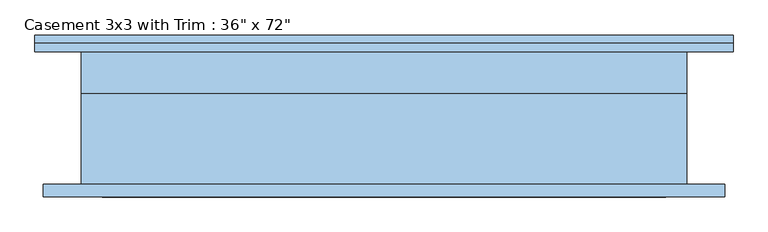
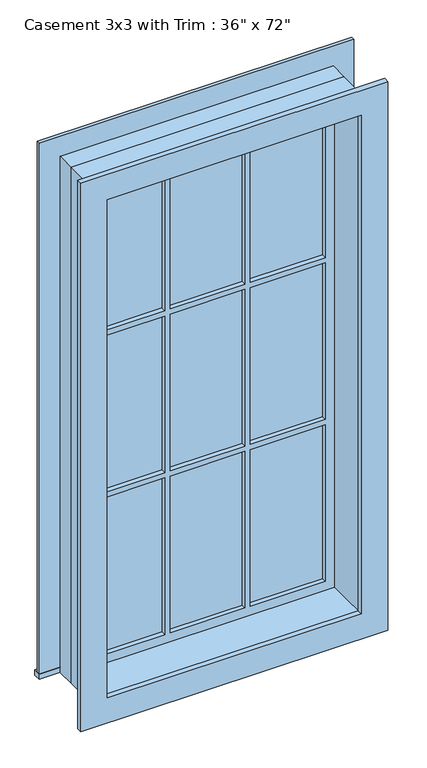
"""IFC4 building model written with IfcOpenShell, lengths in millimetres: window geometry."""

from ifc_helpers import new_model, si_unit, frame, origin, place, context, project, spatial, polyline, outline, extrude, source, transform, mapped, element, save


def window_0c844ac8(model_context):
    return source(origin(), model_context, "Body", "SweptSolid", [
        extrude(outline(polyline([(-527.05, 125.4), (527.05, 125.4), (527.05, 100.0), (-527.05, 100.0), (-527.05, 125.4)])), frame((0.0, 0.0, 304.8), z_axis=(0.0, 0.0, 1.0), x_axis=(1.0, 0.0, 0.0)), (0.0, 0.0, 1.0), 19.05),
        extrude(outline(polyline([(2114.55, -438.15), (2114.55, 438.15), (323.85, 438.15), (323.85, 527.05), (2203.45, 527.05), (2203.45, -527.05), (323.85, -527.05), (323.85, -438.15), (2114.55, -438.15)])), frame((0.0, 100.0, 0.0), z_axis=(0.0, 1.0, 0.0), x_axis=(0.0, 0.0, 1.0)), (0.0, 0.0, 1.0), 12.7),
        extrude(outline(polyline([(143.9333333, 65.075), (393.7, 65.075), (393.7, 52.375), (143.9333333, 52.375), (143.9333333, 65.075)])), frame((0.0, 0.0, 1515.5333333), z_axis=(0.0, 0.0, 1.0), x_axis=(1.0, 0.0, 0.0)), (0.0, 0.0, 1.0), 554.5666667),
        extrude(outline(polyline([(-124.8833333, 65.075), (124.8833333, 65.075), (124.8833333, 52.375), (-124.8833333, 52.375), (-124.8833333, 65.075)])), frame((0.0, 0.0, 1515.5333333), z_axis=(0.0, 0.0, 1.0), x_axis=(1.0, 0.0, 0.0)), (0.0, 0.0, 1.0), 554.5666667),
        extrude(outline(polyline([(-393.7, 65.075), (-143.9333333, 65.075), (-143.9333333, 52.375), (-393.7, 52.375), (-393.7, 65.075)])), frame((0.0, 0.0, 1515.5333333), z_axis=(0.0, 0.0, 1.0), x_axis=(1.0, 0.0, 0.0)), (0.0, 0.0, 1.0), 554.5666667),
        extrude(outline(polyline([(-393.7, 65.075), (-143.9333333, 65.075), (-143.9333333, 52.375), (-393.7, 52.375), (-393.7, 65.075)])), frame((0.0, 0.0, 941.9166667), z_axis=(0.0, 0.0, 1.0), x_axis=(1.0, 0.0, 0.0)), (0.0, 0.0, 1.0), 554.5666667),
        extrude(outline(polyline([(-124.8833333, 65.075), (124.8833333, 65.075), (124.8833333, 52.375), (-124.8833333, 52.375), (-124.8833333, 65.075)])), frame((0.0, 0.0, 941.9166667), z_axis=(0.0, 0.0, 1.0), x_axis=(1.0, 0.0, 0.0)), (0.0, 0.0, 1.0), 554.5666667),
        extrude(outline(polyline([(143.9333333, 65.075), (393.7, 65.075), (393.7, 52.375), (143.9333333, 52.375), (143.9333333, 65.075)])), frame((0.0, 0.0, 941.9166667), z_axis=(0.0, 0.0, 1.0), x_axis=(1.0, 0.0, 0.0)), (0.0, 0.0, 1.0), 554.5666667),
        extrude(outline(polyline([(143.9333333, 65.075), (393.7, 65.075), (393.7, 52.375), (143.9333333, 52.375), (143.9333333, 65.075)])), frame((0.0, 0.0, 368.3), z_axis=(0.0, 0.0, 1.0), x_axis=(1.0, 0.0, 0.0)), (0.0, 0.0, 1.0), 554.5666667),
        extrude(outline(polyline([(-124.8833333, 65.075), (124.8833333, 65.075), (124.8833333, 52.375), (-124.8833333, 52.375), (-124.8833333, 65.075)])), frame((0.0, 0.0, 368.3), z_axis=(0.0, 0.0, 1.0), x_axis=(1.0, 0.0, 0.0)), (0.0, 0.0, 1.0), 554.5666667),
        extrude(outline(polyline([(-393.7, 65.075), (-143.9333333, 65.075), (-143.9333333, 52.375), (-393.7, 52.375), (-393.7, 65.075)])), frame((0.0, 0.0, 368.3), z_axis=(0.0, 0.0, 1.0), x_axis=(1.0, 0.0, 0.0)), (0.0, 0.0, 1.0), 554.5666667),
        extrude(outline(polyline([(2190.75, 514.35), (2190.75, -514.35), (247.65, -514.35), (247.65, 514.35), (2190.75, 514.35)]), holes=[polyline([(2101.85, 425.45), (336.55, 425.45), (336.55, -425.45), (2101.85, -425.45), (2101.85, 425.45)])]), frame((0.0, -119.05, 0.0), z_axis=(0.0, 1.0, 0.0), x_axis=(0.0, 0.0, 1.0)), (0.0, 0.0, 1.0), 19.05),
        extrude(outline(polyline([(2114.55, -438.15), (323.85, -438.15), (323.85, 438.15), (2114.55, 438.15), (2114.55, -438.15)]), holes=[polyline([(2070.1, -143.9333333), (1515.5333333, -143.9333333), (1515.5333333, -393.7), (2070.1, -393.7), (2070.1, -143.9333333)]), polyline([(1496.4833333, -143.9333333), (941.9166667, -143.9333333), (941.9166667, -393.7), (1496.4833333, -393.7), (1496.4833333, -143.9333333)]), polyline([(922.8666667, -143.9333333), (368.3, -143.9333333), (368.3, -393.7), (922.8666667, -393.7), (922.8666667, -143.9333333)]), polyline([(2070.1, 124.8833333), (1515.5333333, 124.8833333), (1515.5333333, -124.8833333), (2070.1, -124.8833333), (2070.1, 124.8833333)]), polyline([(1496.4833333, 124.8833333), (941.9166667, 124.8833333), (941.9166667, -124.8833333), (1496.4833333, -124.8833333), (1496.4833333, 124.8833333)]), polyline([(922.8666667, 124.8833333), (368.3, 124.8833333), (368.3, -124.8833333), (922.8666667, -124.8833333), (922.8666667, 124.8833333)]), polyline([(2070.1, 393.7), (1515.5333333, 393.7), (1515.5333333, 143.9333333), (2070.1, 143.9333333), (2070.1, 393.7)]), polyline([(1496.4833333, 393.7), (941.9166667, 393.7), (941.9166667, 143.9333333), (1496.4833333, 143.9333333), (1496.4833333, 393.7)]), polyline([(922.8666667, 393.7), (368.3, 393.7), (368.3, 143.9333333), (922.8666667, 143.9333333), (922.8666667, 393.7)])]), frame((0.0, 36.5, 0.0), z_axis=(0.0, 1.0, 0.0), x_axis=(0.0, 0.0, 1.0)), (0.0, 0.0, 1.0), 44.45),
        extrude(outline(polyline([(2133.6, -457.2), (304.8, -457.2), (304.8, 457.2), (2133.6, 457.2), (2133.6, -457.2)]), holes=[polyline([(2101.85, -425.45), (2101.85, 425.45), (336.55, 425.45), (336.55, -425.45), (2101.85, -425.45)])]), frame((0.0, -100.0, 0.0), z_axis=(0.0, 1.0, 0.0), x_axis=(0.0, 0.0, 1.0)), (0.0, 0.0, 1.0), 136.5),
        extrude(outline(polyline([(2133.6, 457.2), (2133.6, -457.2), (304.8, -457.2), (304.8, 457.2), (2133.6, 457.2)]), holes=[polyline([(2114.55, 438.15), (323.85, 438.15), (323.85, -438.15), (2114.55, -438.15), (2114.55, 438.15)])]), frame((0.0, 36.5, 0.0), z_axis=(0.0, 1.0, 0.0), x_axis=(0.0, 0.0, 1.0)), (0.0, 0.0, 1.0), 63.5),
    ])


if __name__ == "__main__":
    model = new_model("IFC4")
    model_context = context("Model", 3, world=origin())
    ifc_project = project(units=[si_unit("LENGTHUNIT", "METRE", prefix="MILLI")], contexts=[model_context])
    site = spatial("IfcSite", under=ifc_project)
    building = spatial("IfcBuilding", under=site)
    placement = place(None, origin())
    window_shape = window_0c844ac8(model_context)
    element("IfcWindow", 1, ObjectType="Casement 3x3 with Trim : 36\" x 72\"", at=placement, inside=building, context=model_context, shape_type="MappedRepresentation", body=[
        mapped(window_shape, transform((0.0, 0.0, 0.0), x_axis=(1.0, 0.0, 0.0), y_axis=(0.0, 1.0, 0.0), z_axis=(0.0, 0.0, 1.0))),
    ])
    save(model, "model.ifc")

# Revit data of these elements
# Type "Casement 3x3 with Trim : 36\" x 72\""
#   Type Mark = "21"
#   Construction Type Id = "GSP4R"
#   Assembly Code = "B2020100"
#   Analytic Construction = "1/8 in Pilkington single glazing"
#   Visual Light Transmittance = 0.9
#   Solar Heat Gain Coefficient = 0.78
#   Heat Transfer Coefficient (U) = 3.6886 W/(m²·K)
#   Height = 6' - 0"
#   Default Sill Height = 1' - 0"
#   Trim Projection - Ext. = 0' - 0 1/2"
#   Trim Projection - Int. = 0' - 0 3/4"
#   Trim Width - Exterior = 0' - 3 1/2"
#   Trim Width - Interior = 0' - 3 1/2"
#   Width = 3' - 0"
#   Window Inset = 0' - 0 3/4"
#   Define Thermal Properties by = 1
#   Glass Pane Material = Glass
#   Sash Material = Sash
#   Trim Exterior Material = Trim
#   Trim Interior Material = Trim
#   Wall Closure = (empty or 0)
# Element 1 (IfcWindow, "Casement 3x3 with Trim : 36\" x 72\"")
#   Materials on its faces: "Sash", "Glass", "Trim"
# Materials
#   "Glass": class "Glass", colour RGB 218 227 224, transparency 0.85, Description = "Soda Lime Glass", Cost = 0
#   "Sash": class "Wood", colour RGB 136 99 55, transparency 0
#   "Trim": class "Wood", colour RGB 224 178 126, transparency 0
